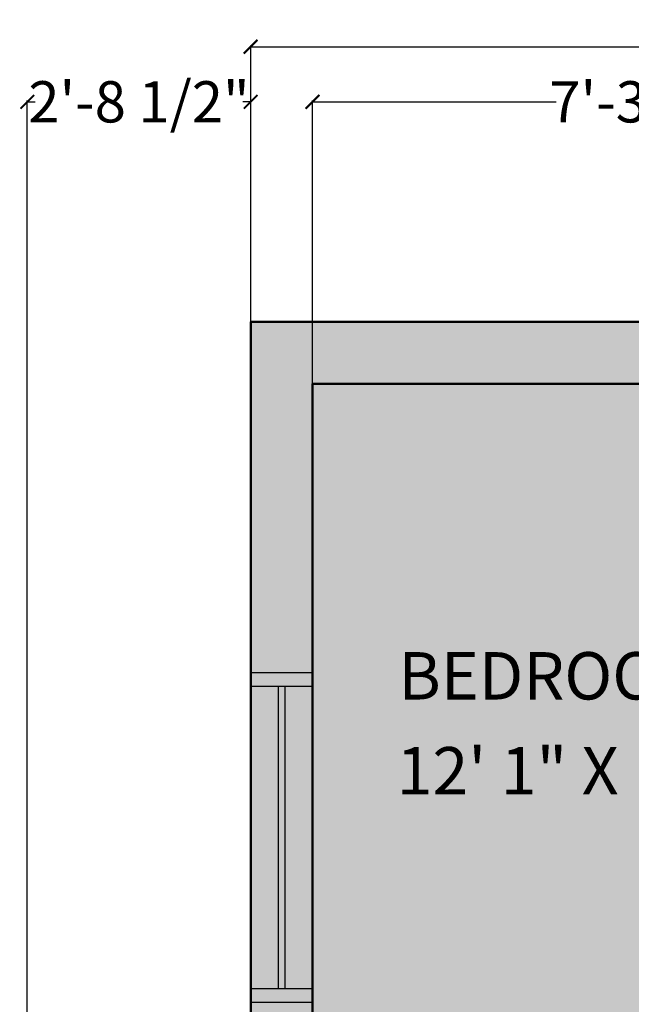
# Model space of a CAD drawing. Units: inches. Extents: x 528 to 2620, y -1066 to 798.
# Tile 26 of 41: x 1023 to 1112, y 620 to 763. Entities that reach past the tile are written whole.
import ezdxf

# ---------------------------------------------------------------- set-up
doc = ezdxf.new("R2010")
doc.units = ezdxf.units.IN
doc.header["$MEASUREMENT"] = 0
for name, color, linetype, lineweight in [('A-ANNO-DIMS', 2, 'Continuous', 18), ('A-AREA-IDEN', 7, 'Continuous', 18), ('A-GLAZ', 3, 'Continuous', 25), ('A-WALL', 7, 'Continuous', 50), ('A-WALL-PATT', 8, 'Continuous', 13)]:
    doc.layers.add(name, color=color, linetype=linetype, lineweight=lineweight)
doc.styles.get("Standard").update_dxf_attribs({"font": 'arial.ttf'})
doc.dimstyles.get("Standard").update_dxf_attribs({"dimtxt": 6, "dimasz": 2, "dimexe": 0.18, "dimexo": 0.0625, "dimgap": 0.09, "dimtad": 0, "dimtih": 1, "dimtoh": 1, "dimdec": 1, "dimzin": 0, "dimdsep": 46, "dimlunit": 3, "dimtxsty": 'Standard', "dimblk": 'ARCHTICK', "dimcen": 0.09, "dimadec": 0, "dimazin": 0, "dimtfac": 1, "dimtdec": 1, "dimtofl": 0, "dimtmove": 0, "dimatfit": 3, "dimfxl": 1, "dimtolj": 1, "dimtzin": 0, "dimarcsym": 0})

# ---------------------------------------------------------------- blocks, each defined once
blk = doc.blocks.new('_ArchTick')
at = {"color": 0, "linetype": 'ByBlock', "const_width": 0.15}
blk.add_lwpolyline([(-0.5, -0.5), (0.5, 0.5)], dxfattribs=at)
blk = doc.blocks.new('*D18')
at = {"layer": 'A-ANNO-DIMS', "color": 0, "lineweight": -2, "transparency": 16777216}
for p, q in [((1057, 718.98), (1057, 759.11)), ((1057, 758.93), (1195.76, 758.93)), ((1345, 758.93), (1206.23, 758.93)), ((1345, 718.98), (1345, 759.11))]:
    blk.add_line(p, q, dxfattribs=at)
at = {"layer": 'Defpoints', "color": 0, "transparency": 16777216}
for p in [(1345, 758.93), (1057, 718.92), (1345, 718.92)]:
    blk.add_point(p, dxfattribs=at)
at = {"layer": 'A-ANNO-DIMS', "color": 0, "lineweight": -2, "transparency": 16777216, "xscale": 2, "yscale": 2, "zscale": 2, "rotation": 180}
blk.add_blockref('_ArchTick', (1057, 758.93), dxfattribs=at)
at = {"layer": 'A-ANNO-DIMS', "color": 0, "lineweight": -2, "transparency": 16777216, "xscale": 2, "yscale": 2, "zscale": 2}
blk.add_blockref('_ArchTick', (1345, 758.93), dxfattribs=at)
at = {"layer": 'A-ANNO-DIMS', "color": 0, "transparency": 16777216, "insert": (1201, 758.93), "char_height": 6, "attachment_point": 5}
blk.add_mtext("\\A1;24'", dxfattribs=at)
blk = doc.blocks.new('WIN-1200')
for p, q in [((677.56, 718.92), (725.56, 718.92)), ((677.56, 709.92), (677.56, 718.92)), ((679.56, 709.92), (679.56, 718.92)), ((723.56, 718.92), (723.56, 709.92)), ((725.56, 718.92), (725.56, 709.92)), ((679.56, 714.92), (723.56, 714.92)), ((679.56, 713.92), (723.56, 713.92)), ((725.56, 709.92), (677.56, 709.92))]:
    blk.add_line(p, q)
blk = doc.blocks.new('*D63')
at = {"layer": 'A-ANNO-DIMS', "color": 0, "lineweight": -2, "transparency": 16777216}
for p, q in [((1024.5, 405.4), (1024.5, 751.1)), ((1024.5, 750.92), (1025.64, 750.92)), ((1057, 750.92), (1055.85, 750.92)), ((1057, 405.4), (1057, 751.1))]:
    blk.add_line(p, q, dxfattribs=at)
at = {"layer": 'Defpoints', "color": 0, "transparency": 16777216}
for p in [(1057, 750.92), (1024.5, 405.34), (1057, 405.34)]:
    blk.add_point(p, dxfattribs=at)
at = {"layer": 'A-ANNO-DIMS', "color": 0, "lineweight": -2, "transparency": 16777216, "xscale": 2, "yscale": 2, "zscale": 2, "rotation": 180}
blk.add_blockref('_ArchTick', (1024.5, 750.92), dxfattribs=at)
at = {"layer": 'A-ANNO-DIMS', "color": 0, "lineweight": -2, "transparency": 16777216, "xscale": 2, "yscale": 2, "zscale": 2}
blk.add_blockref('_ArchTick', (1057, 750.92), dxfattribs=at)
at = {"layer": 'A-ANNO-DIMS', "color": 0, "transparency": 16777216, "insert": (1040.75, 750.92), "char_height": 6, "attachment_point": 5}
blk.add_mtext('\\A1;2\'-8 1/2"', dxfattribs=at)
blk = doc.blocks.new('*D66')
at = {"layer": 'A-ANNO-DIMS', "color": 0, "lineweight": -2, "transparency": 16777216}
for p, q in [((1066, 400.48), (1066, 751.1)), ((1066, 750.92), (1101.46, 750.92)), ((1153, 750.92), (1117.54, 750.92)), ((1153, 400.48), (1153, 751.1))]:
    blk.add_line(p, q, dxfattribs=at)
at = {"layer": 'Defpoints', "color": 0, "transparency": 16777216}
for p in [(1153, 750.92), (1066, 400.42), (1153, 400.42)]:
    blk.add_point(p, dxfattribs=at)
at = {"layer": 'A-ANNO-DIMS', "color": 0, "lineweight": -2, "transparency": 16777216, "xscale": 2, "yscale": 2, "zscale": 2, "rotation": 180}
blk.add_blockref('_ArchTick', (1066, 750.92), dxfattribs=at)
at = {"layer": 'A-ANNO-DIMS', "color": 0, "lineweight": -2, "transparency": 16777216, "xscale": 2, "yscale": 2, "zscale": 2}
blk.add_blockref('_ArchTick', (1153, 750.92), dxfattribs=at)
at = {"layer": 'A-ANNO-DIMS', "color": 0, "transparency": 16777216, "insert": (1109.5, 750.92), "char_height": 6, "attachment_point": 5}
blk.add_mtext('\\A1;7\'-3"', dxfattribs=at)

msp = doc.modelspace()

# ---------------------------------------------------------------- hatches: boundary and pattern name
at = {"layer": 'A-WALL-PATT', "transparency": 33554521}
h = msp.add_hatch(color=256, dxfattribs=at)
h.dxf.hatch_style = 1
h.paths.add_polyline_path([(1066, 709.92), (1114.5, 709.92), (1114.5, 718.92), (1057, 718.92), (1057, 667.92), (1066, 667.92)])
h.paths.add_polyline_path([(1227.5, 718.92), (1162.5, 718.92), (1162.5, 709.92), (1211, 709.92), (1211, 577.92), (1205.42, 577.92), (1205.5, 573.42), (1211, 573.42), (1211, 567.42), (1215.5, 567.42), (1215.5, 669.42), (1268, 669.42), (1268, 675.92), (1263.5, 675.92), (1263.5, 673.92), (1215.5, 673.92), (1215.5, 709.92), (1227.5, 709.92)])
h.paths.add_polyline_path([(1345, 718.92), (1316, 718.92), (1316, 709.92), (1336, 709.92), (1336, 641.67), (1345, 641.67)])
h.paths.add_polyline_path([(1066, 619.92), (1057, 619.92), (1057, 561.42), (1066, 561.42), (1066, 573.42), (1161, 573.42), (1161, 569.42), (1165.5, 569.42), (1165.5, 577.92), (1066, 577.92)])
h.paths.add_polyline_path([(1216, 391.42), (1216, 400.42), (1207, 400.42), (1201, 400.42), (1201, 397.42), (1201, 391.42), (1207, 391.42), (1207, 268.92), (1252, 268.92), (1252, 277.92), (1216, 277.92), (1216, 359.77)])
h.paths.add_polyline_path([(1345, 395.92), (1336, 395.92), (1288, 395.92), (1288, 391.42), (1336, 391.42), (1336, 277.92), (1300, 277.92), (1300, 268.92), (1345, 268.92)])
h.paths.add_polyline_path([(1345, 593.67), (1336, 593.67), (1336, 525.42), (1215.5, 525.42), (1215.5, 527.17), (1211, 527.17), (1211, 520.92), (1336, 520.92), (1336, 443.92), (1345, 443.92)])
h.paths.add_polyline_path([(1066, 520.92), (1165.5, 520.92), (1165.5, 545.42), (1161, 545.42), (1161, 525.42), (1066, 525.42), (1066, 537.42), (1057, 537.42), (1057, 484.67), (1066, 484.67)])
h.paths.add_polyline_path([(1066, 436.67), (1057, 436.67), (1057, 391.42), (1085.5, 391.42), (1085.5, 400.42), (1066, 400.42)])
h.paths.add_polyline_path([(1153, 397.42), (1153, 400.42), (1133.5, 400.42), (1133.5, 391.42), (1153, 391.42)])
at = {"layer": 'A-WALL-PATT', "transparency": 33554681}
h = msp.add_hatch(color=256, dxfattribs=at)
h.dxf.hatch_style = 1
h.paths.add_polyline_path([(1062, 665.92), (1061, 665.92), (1061, 621.92), (1062, 621.92)])
h.paths.add_polyline_path([(1066, 667.92), (1057, 667.92), (1057, 665.92), (1066, 665.92)])
h.paths.add_polyline_path([(1066, 621.92), (1057, 621.92), (1057, 619.92), (1066, 619.92)])
h.paths.add_polyline_path([(1160.5, 714.92), (1116.5, 714.92), (1116.5, 713.92), (1160.5, 713.92)])
h.paths.add_polyline_path([(1162.5, 718.92), (1160.5, 718.92), (1160.5, 709.92), (1162.5, 709.92)])
h.paths.add_polyline_path([(1116.5, 718.92), (1114.5, 718.92), (1114.5, 709.92), (1116.5, 709.92)])
h.paths.add_polyline_path([(1251.5, 714.92), (1227.5, 714.92), (1227.5, 713.92), (1251.5, 713.92)])
h.paths.add_polyline_path([(1314, 714.92), (1270, 714.92), (1270, 713.92), (1314, 713.92)])
h.paths.add_polyline_path([(1316, 718.92), (1314, 718.92), (1314, 709.92), (1316, 709.92)])
h.paths.add_polyline_path([(1270, 718.92), (1268, 718.92), (1268, 709.92), (1270, 709.92)])
h.paths.add_polyline_path([(1087.5, 400.42), (1085.5, 400.42), (1085.5, 391.42), (1087.5, 391.42)])
h.paths.add_polyline_path([(1131.5, 396.42), (1087.5, 396.42), (1087.5, 395.42), (1131.5, 395.42)])
h.paths.add_polyline_path([(1133.5, 400.42), (1131.5, 400.42), (1131.5, 391.42), (1133.5, 391.42)])
h.paths.add_polyline_path([(1066, 438.67), (1057, 438.67), (1057, 436.67), (1066, 436.67)])
h.paths.add_polyline_path([(1066, 484.67), (1057, 484.67), (1057, 482.67), (1066, 482.67)])
h.paths.add_polyline_path([(1062, 482.67), (1061, 482.67), (1061, 438.67), (1062, 438.67)])
h = msp.add_hatch(color=256, dxfattribs=at)
h.dxf.hatch_style = 1
h.paths.add_polyline_path([(1066, 665.92), (1062, 665.92), (1062, 621.92), (1066, 621.92)])
h.paths.add_polyline_path([(1061, 665.92), (1057, 665.92), (1057, 621.92), (1061, 621.92)])
h.paths.add_polyline_path([(1160.5, 713.92), (1116.5, 713.92), (1116.5, 709.92), (1160.5, 709.92)])
h.paths.add_polyline_path([(1160.5, 718.92), (1116.5, 718.92), (1116.5, 714.92), (1160.5, 714.92)])
h.paths.add_polyline_path([(1251.5, 713.92), (1227.5, 713.92), (1227.5, 709.92), (1251.5, 709.92)])
h.paths.add_polyline_path([(1251.5, 718.92), (1227.5, 718.92), (1227.5, 714.92), (1251.5, 714.92)])
h.paths.add_polyline_path([(1314, 713.92), (1270, 713.92), (1270, 709.92), (1314, 709.92)])
h.paths.add_polyline_path([(1314, 718.92), (1270, 718.92), (1270, 714.92), (1314, 714.92)])
h.paths.add_polyline_path([(1345, 639.67), (1341, 639.67), (1341, 595.67), (1345, 595.67)])
h.paths.add_polyline_path([(1340, 639.67), (1336, 639.67), (1336, 595.67), (1340, 595.67)])
h.paths.add_polyline_path([(1345, 441.92), (1341, 441.92), (1341, 397.92), (1345, 397.92)])
h.paths.add_polyline_path([(1340, 441.92), (1336, 441.92), (1336, 397.92), (1340, 397.92)])
h.paths.add_polyline_path([(1298, 272.92), (1254, 272.92), (1254, 268.92), (1298, 268.92)])
h.paths.add_polyline_path([(1298, 277.92), (1254, 277.92), (1254, 273.92), (1298, 273.92)])
h.paths.add_polyline_path([(1131.5, 395.42), (1087.5, 395.42), (1087.5, 391.42), (1131.5, 391.42)])
h.paths.add_polyline_path([(1131.5, 400.42), (1087.5, 400.42), (1087.5, 396.42), (1131.5, 396.42)])
h.paths.add_polyline_path([(1066, 482.67), (1062, 482.67), (1062, 438.67), (1066, 438.67)])
h.paths.add_polyline_path([(1061, 482.67), (1057, 482.67), (1057, 438.67), (1061, 438.67)])
h.paths.add_polyline_path([(1066, 561.42), (1062, 561.42), (1062, 537.42), (1066, 537.42)])
h.paths.add_polyline_path([(1061, 561.42), (1057, 561.42), (1057, 537.42), (1061, 537.42)])
at = {"layer": 'A-WALL-PATT', "transparency": 33554536}
h = msp.add_hatch(color=256, dxfattribs=at)
h.dxf.hatch_style = 1
h.paths.add_polyline_path([(1336, 709.92), (1268, 709.92), (1268, 699.92), (1266.75, 699.92), (1266.75, 675.92), (1268, 675.92), (1268, 669.42), (1215.5, 669.42), (1215.5, 567.17), (1217, 567.17), (1257, 567.17), (1257, 565.42), (1256.96, 565.42, -0.401453), (1217, 527.17), (1215.5, 527.17), (1215.5, 525.42), (1336, 525.42)], flags=17)
h.paths.add_polyline_path([(1285.03, 635.93), (1285.23, 636.13), (1285.67, 636.26), (1286.21, 636.02), (1286.98, 636.08), (1332.98, 636.08), (1333.36, 636.22), (1333.82, 636.08), (1334.11, 635.71), (1334.11, 635.3), (1333.91, 634.86), (1333.82, 634.83), (1333.82, 592.74), (1333.97, 592.6), (1334.11, 592.29), (1334.11, 591.88), (1333.82, 591.51), (1333.36, 591.37), (1332.98, 591.51), (1332.64, 591.79), (1332.64, 591.51), (1286.98, 591.51), (1286.17, 591.67), (1286.07, 591.57), (1285.68, 591.37), (1285.23, 591.51), (1285.03, 591.71), (1284.83, 592.1), (1284.98, 592.54), (1285.13, 592.69), (1285.13, 634.95), (1284.98, 635.1), (1284.83, 635.54)], flags=16)
h.paths.add_polyline_path([(1285.03, 635.93), (1285.23, 636.13), (1285.67, 636.26), (1286.21, 636.02), (1286.98, 636.08), (1332.98, 636.08), (1333.36, 636.22), (1333.82, 636.08), (1334.11, 635.71), (1334.11, 635.3), (1333.97, 634.99), (1333.82, 634.85), (1333.82, 592.74), (1333.97, 592.6), (1334.11, 592.29), (1334.11, 591.88), (1333.82, 591.51), (1333.36, 591.37), (1332.98, 591.51), (1332.64, 591.79), (1332.64, 592.25), (1332.64, 635.35), (1332.64, 635.8), (1332.98, 636.08), (1312.23, 636.08), (1311.1, 635.48), (1310.63, 635.48), (1310.43, 635.23), (1309.94, 635.1), (1309.7, 634.99), (1309.06, 634.76), (1308.71, 634.61), (1308.32, 634.61), (1307.75, 634.36), (1307.11, 634.27), (1307.01, 634.11), (1306.77, 634.02), (1307.25, 633.28), (1306.87, 633.04), (1306.77, 632.88), (1306.37, 632.64), (1306.03, 632.55), (1305.54, 632.41), (1315.47, 618.49), (1316.32, 619.39), (1312.77, 622.86), (1319.62, 630.11), (1320.07, 629.68), (1320.11, 630), (1320.28, 630.6), (1320.53, 631.18), (1320.53, 632.01), (1320.26, 632.55), (1320.11, 633.13), (1320.06, 633.73), (1320.63, 634.02), (1321.22, 634.16), (1321.86, 634.11), (1322.45, 633.91), (1322.99, 633.62), (1324.1, 633.62), (1324.64, 633.91), (1325.23, 634.07), (1325.87, 634.07), (1326.43, 633.91), (1326.98, 633.62), (1328.35, 633.62), (1328.9, 633.91), (1329.49, 634.11), (1330.1, 634.16), (1330.69, 634.02), (1331.28, 633.73), (1331.23, 633.13), (1331.09, 632.55), (1330.79, 632.01), (1330.79, 631.18), (1331.04, 630.6), (1331.23, 630), (1331.28, 629.41), (1331.19, 628.79), (1331.04, 628.18), (1330.79, 627.6), (1330.79, 626.77), (1331.04, 626.19), (1331.23, 625.59), (1331.28, 625.01), (1331.19, 624.38), (1331.04, 623.78), (1330.79, 623.24), (1330.79, 622.37), (1331.04, 621.83), (1331.23, 621.25), (1331.28, 620.6), (1331.19, 619.97), (1331.04, 619.37), (1330.79, 618.83), (1330.79, 617.96), (1331.09, 617.42), (1331.23, 616.88), (1331.28, 616.23), (1331.28, 615.52), (1330.69, 615.27), (1330.1, 615.12), (1329.49, 615.12), (1328.9, 615.32), (1328.35, 615.65), (1326.98, 615.65), (1326.43, 615.32), (1325.87, 615.16), (1325.23, 615.16), (1324.64, 615.32), (1324.1, 615.65), (1323.24, 615.65), (1324.93, 614.04), (1322.98, 611.98), (1324.1, 611.98), (1324.64, 612.27), (1325.28, 612.43), (1325.87, 612.43), (1326.48, 612.27), (1327.03, 611.98), (1328.35, 611.98), (1328.9, 612.27), (1329.49, 612.48), (1330.1, 612.52), (1330.74, 612.39), (1331.28, 612.07), (1331.28, 611.36), (1331.28, 610.75), (1331.09, 610.17), (1330.79, 609.63), (1330.79, 608.81), (1331.09, 608.22), (1331.23, 607.62), (1331.28, 606.99), (1331.23, 606.41), (1331.09, 605.81), (1330.79, 605.22), (1330.79, 604.4), (1331.09, 603.81), (1331.23, 603.21), (1331.28, 602.63), (1331.23, 602), (1331.09, 601.4), (1330.79, 600.86), (1330.79, 599.99), (1331.09, 599.45), (1331.23, 598.87), (1331.28, 598.22), (1331.23, 597.59), (1331.09, 596.99), (1330.79, 596.45), (1330.79, 595.58), (1331.09, 595.04), (1331.28, 594.51), (1331.28, 593.86), (1330.74, 593.61), (1330.1, 593.48), (1329.49, 593.48), (1328.9, 593.68), (1328.35, 594.01), (1327.03, 594.01), (1326.48, 593.68), (1325.87, 593.52), (1325.28, 593.52), (1324.64, 593.68), (1324.1, 594.01), (1323.04, 594.01), (1322.5, 593.68), (1321.91, 593.48), (1321.27, 593.48), (1320.63, 593.61), (1320.11, 593.86), (1320.11, 594.51), (1320.28, 595.04), (1320.58, 595.58), (1320.58, 596.45), (1320.28, 596.99), (1320.16, 597.59), (1320.1, 598.01), (1319.62, 597.55), (1315.66, 601.73), (1312.23, 591.57), (1311.74, 591.66), (1311.59, 591.91), (1310.78, 592.4), (1309.55, 592.89), (1308.96, 592.89), (1308.71, 593.03), (1308.56, 593.14), (1307.75, 593.52), (1306.77, 593.61), (1307.25, 594.36), (1306.87, 594.6), (1306.37, 594.84), (1306.03, 595.09), (1305.54, 595.24), (1315.46, 609.35), (1310.93, 613.71), (1315.47, 618.49), (1305.54, 632.41), (1306.03, 632.55), (1306.37, 632.64), (1306.77, 632.88), (1306.87, 633.04), (1307.25, 633.28), (1306.77, 634.02), (1307.01, 634.11), (1307.11, 634.27), (1307.75, 634.36), (1308.32, 634.61), (1308.71, 634.61), (1309.06, 634.76), (1309.7, 634.99), (1309.94, 635.1), (1310.43, 635.23), (1310.63, 635.48), (1311.1, 635.48), (1312.23, 636.08), (1286.98, 636.08), (1286.22, 636.02), (1286.41, 635.44), (1286.21, 635.05), (1286.02, 634.85), (1285.87, 634.81), (1285.87, 592.84), (1286.15, 592.73), (1286.41, 592.19), (1286.23, 591.66), (1286.17, 591.67), (1286.07, 591.57), (1285.68, 591.37), (1285.23, 591.51), (1285.03, 591.71), (1284.83, 592.1), (1284.98, 592.54), (1285.13, 592.69), (1285.13, 634.95), (1284.98, 635.1), (1284.83, 635.54)], flags=0)
h.paths.add_polyline_path([(1322.5, 653.6), (1333.65, 653.6), (1333.65, 637.99), (1322.5, 637.99)], flags=16)
h.paths.add_polyline_path([(1323.62, 652.48), (1332.53, 652.48), (1332.53, 639.11), (1323.62, 639.11)], flags=0)
edge = h.paths.add_edge_path(flags=0)
edge.add_ellipse((1328.07, 645.79), major_axis=(2.24, 2.24), ratio=1, start_angle=405, end_angle=495, ccw=False)
edge.add_ellipse((1328.07, 645.79), major_axis=(2.24, 2.24), ratio=1, start_angle=675, end_angle=765, ccw=False)
edge.add_ellipse((1328.07, 645.79), major_axis=(2.24, 2.24), ratio=1, start_angle=585, end_angle=675, ccw=False)
edge.add_ellipse((1328.07, 645.79), major_axis=(2.24, 2.24), ratio=1, start_angle=495, end_angle=585, ccw=False)
h.paths.add_polyline_path([(1320.58, 628.39), (1320.33, 628.01), (1320.61, 628.55)], flags=0)
h.paths.add_polyline_path([(1317.89, 604.89), (1318.78, 604.64), (1319.76, 604.28), (1318.88, 604.53)], flags=0)
h.paths.add_polyline_path([(1320.33, 599.65), (1320.58, 599.25), (1320.58, 599.16)], flags=0)
h.paths.add_polyline_path([(1322.5, 589.6), (1333.65, 589.6), (1333.65, 573.99), (1322.5, 573.99)], flags=16)
h.paths.add_polyline_path([(1323.62, 588.48), (1332.53, 588.48), (1332.53, 575.11), (1323.62, 575.11)], flags=0)
edge = h.paths.add_edge_path(flags=0)
edge.add_ellipse((1328.07, 581.8), major_axis=(-2.24, 2.24), ratio=1, start_angle=-45, end_angle=45, ccw=False)
edge.add_ellipse((1328.07, 581.8), major_axis=(-2.24, 2.24), ratio=1, start_angle=-135, end_angle=-45, ccw=False)
edge.add_ellipse((1328.07, 581.8), major_axis=(-2.24, 2.24), ratio=1, start_angle=135, end_angle=-135, ccw=False)
edge.add_ellipse((1328.07, 581.8), major_axis=(-2.24, 2.24), ratio=1, start_angle=45, end_angle=135, ccw=False)
h.paths.add_polyline_path([(1264.75, 699.92), (1263.5, 699.92), (1263.5, 709.92), (1215.5, 709.92), (1215.5, 673.92), (1263.5, 673.92), (1263.5, 675.92), (1264.75, 675.92)], flags=16)
h.paths.add_polyline_path([(1162.19, 569.42), (1161, 569.42), (1161, 573.42), (1066, 573.42), (1066, 525.42), (1161, 525.42), (1161, 545.42), (1162.19, 545.42)])
h.paths.add_polyline_path([(1256.96, 565.42), (1257, 565.42), (1257, 567.17), (1217, 567.17), (1215.5, 567.17), (1215.5, 567.42), (1211, 567.42), (1211, 573.42), (1205.5, 573.42), (1205.42, 577.92), (1211, 577.92), (1211, 709.92), (1066, 709.92), (1066, 577.92), (1165.5, 577.92), (1165.5, 569.42), (1164.19, 569.42), (1164.19, 545.42), (1165.5, 545.42), (1165.5, 520.92), (1153, 520.92), (1153, 484.92), (1102, 484.92), (1102, 436.42), (1153, 436.42), (1153, 400.42), (1153, 391.42), (1201, 391.42), (1201, 400.42), (1207, 400.42), (1216, 400.42), (1216, 391.42), (1216, 277.92), (1336, 277.92), (1336, 391.42), (1288, 391.42), (1288, 395.92), (1336, 395.92), (1336, 443.92), (1336, 520.92), (1211, 520.92), (1211, 527.17), (1215.5, 527.17), (1217, 527.17, 0.401453)])
h.paths.add_polyline_path([(1167.25, 579.42), (1165.5, 579.42), (1165.5, 619.42), (1167.25, 619.42)], flags=16)
h.paths.add_polyline_path([(1227.97, 501.56), (1236.36, 502.03), (1236.36, 492.55), (1227.97, 493.02, -0.254069)], flags=16)
h.paths.add_polyline_path([(1243.34, 515.69, -0.254069), (1251.88, 515.69), (1252.35, 507.3), (1242.87, 507.3)], flags=16)
h.paths.add_polyline_path([(1239.18, 504.68), (1256.03, 504.68), (1256.03, 479.42), (1239.18, 479.42)], flags=16)
h.paths.add_polyline_path([(1227.97, 489.6), (1236.36, 490.07), (1236.36, 480.59), (1227.97, 481.06, -0.254069)], flags=16)
h.paths.add_polyline_path([(1197.2, 624.04), (1197.2, 639.64), (1208.35, 639.64), (1208.35, 624.04)], flags=16)
h.paths.add_polyline_path([(1198.32, 625.15), (1198.32, 638.53), (1207.23, 638.53), (1207.23, 625.15)], flags=0)
h.paths.add_polyline_path([(1258.85, 502.03), (1267.25, 501.56, -0.254069), (1267.25, 493.02), (1258.85, 492.55)], flags=16)
h.paths.add_polyline_path([(1271.59, 519.66), (1333.67, 519.66), (1333.67, 451.59), (1319.09, 451.59), (1319.09, 505.07), (1288.09, 505.07), (1284.45, 505.07, -0.883215), (1270.68, 514.19), (1270.68, 518.75, -0.414214)], flags=16)
h.paths.add_polyline_path([(1331.85, 517.83), (1331.85, 453.42), (1328.2, 453.42), (1328.2, 505.07), (1298.42, 505.07), (1298.42, 514.19), (1288.09, 514.19), (1288.09, 517.83)], flags=0)
h.paths.add_polyline_path([(1242.87, 476.8), (1252.35, 476.8), (1251.88, 468.41, -0.254069), (1243.34, 468.41)], flags=16)
h.paths.add_polyline_path([(1258.85, 490.07), (1267.25, 489.6, -0.254069), (1267.25, 481.06), (1258.85, 480.59)], flags=16)
h.paths.add_polyline_path([(1161.68, 641.55), (1160.87, 641.72), (1160.77, 641.62), (1160.38, 641.41), (1159.93, 641.55), (1159.73, 641.75), (1159.53, 642.14), (1159.68, 642.58), (1159.83, 642.73), (1159.83, 684.99), (1159.68, 685.14), (1159.53, 685.58), (1159.73, 685.97), (1159.93, 686.17), (1160.37, 686.31), (1160.91, 686.06), (1161.68, 686.13), (1207.68, 686.13), (1208.06, 686.27), (1208.52, 686.13), (1208.81, 685.76), (1208.81, 685.34), (1208.61, 684.9), (1208.52, 684.87), (1208.52, 642.78), (1208.67, 642.65), (1208.88, 642.2), (1208.72, 641.8), (1208.52, 641.55), (1208.06, 641.41), (1207.68, 641.55), (1207.34, 641.83), (1207.34, 641.55)], flags=16)
h.paths.add_polyline_path([(1186.93, 641.62), (1186.44, 641.71), (1186.29, 641.95), (1185.48, 642.45), (1184.25, 642.94), (1183.66, 642.94), (1183.41, 643.07), (1183.26, 643.18), (1182.45, 643.57), (1181.47, 643.65), (1181.95, 644.4), (1181.57, 644.64), (1181.07, 644.89), (1180.73, 645.13), (1180.24, 645.29), (1190.16, 659.4), (1185.63, 663.75), (1190.17, 668.54), (1180.24, 682.46), (1180.73, 682.59), (1181.07, 682.68), (1181.47, 682.93), (1181.57, 683.08), (1181.95, 683.33), (1181.47, 684.07), (1181.71, 684.16), (1181.81, 684.31), (1182.45, 684.4), (1183.02, 684.65), (1183.41, 684.65), (1183.76, 684.81), (1184.4, 685.03), (1184.64, 685.14), (1185.13, 685.28), (1185.33, 685.52), (1185.8, 685.52), (1186.93, 686.13), (1161.68, 686.13), (1160.92, 686.06), (1161.11, 685.49), (1160.91, 685.1), (1160.72, 684.9), (1160.57, 684.85), (1160.57, 642.88), (1160.85, 642.77), (1161.11, 642.23), (1160.93, 641.7), (1160.87, 641.72), (1160.77, 641.62), (1160.38, 641.41), (1159.93, 641.55), (1159.73, 641.75), (1159.53, 642.14), (1159.68, 642.58), (1159.83, 642.73), (1159.83, 684.99), (1159.68, 685.14), (1159.53, 685.58), (1159.73, 685.97), (1159.93, 686.17), (1160.37, 686.31), (1160.91, 686.06), (1161.68, 686.13), (1207.68, 686.13), (1208.06, 686.27), (1208.52, 686.13), (1208.81, 685.76), (1208.81, 685.34), (1208.67, 685.03), (1208.52, 684.9), (1208.52, 642.78), (1208.67, 642.65), (1208.88, 642.2), (1208.72, 641.8), (1208.52, 641.55), (1208.06, 641.41), (1207.68, 641.55), (1207.34, 641.83), (1207.34, 642.29), (1207.34, 685.39), (1207.34, 685.85), (1207.68, 686.13), (1186.93, 686.13), (1185.8, 685.52), (1185.33, 685.52), (1185.13, 685.28), (1184.64, 685.14), (1184.4, 685.03), (1183.76, 684.81), (1183.41, 684.65), (1183.02, 684.65), (1182.45, 684.4), (1181.81, 684.31), (1181.71, 684.16), (1181.47, 684.07), (1181.95, 683.33), (1181.57, 683.08), (1181.47, 682.93), (1181.07, 682.68), (1180.73, 682.59), (1180.24, 682.46), (1190.17, 668.54), (1191.02, 669.43), (1187.47, 672.9), (1194.32, 680.15), (1194.77, 679.72), (1194.81, 680.04), (1194.98, 680.65), (1195.23, 681.23), (1195.23, 682.05), (1194.96, 682.59), (1194.81, 683.17), (1194.76, 683.78), (1195.33, 684.07), (1195.92, 684.2), (1196.56, 684.16), (1197.15, 683.96), (1197.69, 683.67), (1198.8, 683.67), (1199.34, 683.96), (1199.93, 684.11), (1200.57, 684.11), (1201.13, 683.96), (1201.68, 683.67), (1203.05, 683.67), (1203.6, 683.96), (1204.19, 684.16), (1204.8, 684.2), (1205.39, 684.07), (1205.98, 683.78), (1205.93, 683.17), (1205.79, 682.59), (1205.49, 682.05), (1205.49, 681.23), (1205.74, 680.65), (1205.93, 680.04), (1205.98, 679.46), (1205.89, 678.83), (1205.74, 678.23), (1205.49, 677.65), (1205.49, 676.82), (1205.74, 676.24), (1205.93, 675.63), (1205.98, 675.05), (1205.89, 674.42), (1205.74, 673.82), (1205.49, 673.28), (1205.49, 672.41), (1205.74, 671.87), (1205.93, 671.29), (1205.98, 670.64), (1205.89, 670.02), (1205.74, 669.41), (1205.49, 668.87), (1205.49, 668), (1205.79, 667.46), (1205.93, 666.93), (1205.98, 666.28), (1205.98, 665.56), (1205.39, 665.32), (1204.8, 665.16), (1204.19, 665.16), (1203.6, 665.36), (1203.05, 665.7), (1201.68, 665.7), (1201.13, 665.36), (1200.57, 665.2), (1199.93, 665.2), (1199.34, 665.36), (1198.8, 665.7), (1197.94, 665.7), (1199.63, 664.09), (1197.68, 662.03), (1198.8, 662.03), (1199.34, 662.32), (1199.98, 662.47), (1200.57, 662.47), (1201.18, 662.32), (1201.73, 662.03), (1203.05, 662.03), (1203.6, 662.32), (1204.19, 662.52), (1204.8, 662.56), (1205.44, 662.43), (1205.98, 662.12), (1205.98, 661.4), (1205.98, 660.8), (1205.79, 660.21), (1205.49, 659.68), (1205.49, 658.85), (1205.79, 658.27), (1205.93, 657.66), (1205.98, 657.04), (1205.93, 656.45), (1205.79, 655.85), (1205.49, 655.27), (1205.49, 654.44), (1205.79, 653.86), (1205.93, 653.25), (1205.98, 652.67), (1205.93, 652.05), (1205.79, 651.44), (1205.49, 650.91), (1205.49, 650.03), (1205.79, 649.5), (1205.93, 648.91), (1205.98, 648.26), (1205.93, 647.64), (1205.79, 647.03), (1205.49, 646.5), (1205.49, 645.62), (1205.79, 645.09), (1205.98, 644.55), (1205.98, 643.9), (1205.44, 643.65), (1204.8, 643.52), (1204.19, 643.52), (1203.6, 643.72), (1203.05, 644.06), (1201.73, 644.06), (1201.18, 643.72), (1200.57, 643.57), (1199.98, 643.57), (1199.34, 643.72), (1198.8, 644.06), (1197.74, 644.06), (1197.2, 643.72), (1196.61, 643.52), (1195.97, 643.52), (1195.33, 643.65), (1194.81, 643.9), (1194.81, 644.55), (1194.98, 645.09), (1195.28, 645.62), (1195.28, 646.5), (1194.98, 647.03), (1194.86, 647.64), (1194.8, 648.06), (1194.32, 647.59), (1190.36, 651.77)], flags=16)
h.paths.add_polyline_path([(1195.28, 649.2), (1195.03, 649.7), (1195.28, 649.29)], flags=0)
h.paths.add_polyline_path([(1194.46, 654.33), (1193.58, 654.58), (1192.59, 654.93), (1193.48, 654.69)], flags=0)
h.paths.add_polyline_path([(1195.28, 678.43), (1195.03, 678.05), (1195.31, 678.59)], flags=0)
h.paths.add_polyline_path([(1197.2, 688.04), (1197.2, 703.64), (1208.35, 703.64), (1208.35, 688.04)], flags=16)
h.paths.add_polyline_path([(1198.32, 689.15), (1198.32, 702.53), (1207.23, 702.53), (1207.23, 689.15)], flags=0)
h.paths.add_polyline_path([(1217.1, 329.02), (1230.65, 329.02), (1230.65, 315.47), (1217.1, 315.47)], flags=16)
h.paths.add_polyline_path([(1223.87, 322.24), (1227.26, 322.24), (1227.26, 321.32, -0.414214), (1229.73, 318.86, -1), (1224.8, 318.86), (1223.87, 318.86)], flags=0)
h.paths.add_polyline_path([(1222.11, 325.63, -1), (1218.86, 325.63, -1)], flags=0)
h.paths.add_polyline_path([(1228.25, 325.63, -1), (1226.28, 325.63, -1)], flags=0)
h.paths.add_polyline_path([(1221.53, 318.86, -1), (1219.44, 318.86, -1)], flags=0)
h.paths.add_polyline_path([(1299.15, 293.73), (1299.15, 278.54), (1271.23, 278.54), (1271.23, 293.73)], flags=16)
h.paths.add_polyline_path([(1259.69, 292.21), (1270.62, 292.21, -1), (1270.62, 291.6), (1259.69, 291.6, -1)], flags=16)
h.paths.add_polyline_path([(1259.69, 291.3), (1270.62, 291.3, -1), (1270.62, 290.69), (1259.69, 290.69, -1)], flags=16)
h.paths.add_polyline_path([(1259.69, 290.39), (1270.62, 290.39, -1), (1270.62, 289.78), (1259.69, 289.78, -1)], flags=16)
h.paths.add_polyline_path([(1259.69, 289.48), (1270.62, 289.48, -1), (1270.62, 288.87), (1259.69, 288.87, -1)], flags=16)
h.paths.add_polyline_path([(1259.69, 288.57), (1270.62, 288.57, -1), (1270.62, 287.96), (1259.69, 287.96, -1)], flags=16)
h.paths.add_polyline_path([(1274.41, 292.38), (1283.25, 292.38, -0.414214), (1285.07, 290.56), (1285.07, 283.64, -0.414214), (1283.25, 281.82), (1277.72, 281.82), (1278.67, 280.87, -0.57735), (1279.38, 280.16), (1279.44, 280.11, -1), (1279.03, 279.7), (1278.97, 279.75, -0.57735), (1278.26, 280.46), (1276.9, 281.82), (1274.41, 281.82, -0.414214), (1272.58, 283.64), (1272.58, 290.56, -0.414214)], flags=0)
h.paths.add_polyline_path([(1259.69, 287.65), (1270.62, 287.65, -1), (1270.62, 287.05), (1259.69, 287.05, -1)], flags=16)
h.paths.add_polyline_path([(1259.69, 286.74), (1270.62, 286.74, -1), (1270.62, 286.14), (1259.69, 286.14, -1)], flags=16)
h.paths.add_polyline_path([(1259.69, 285.83), (1270.62, 285.83, -1), (1270.62, 285.22), (1259.69, 285.22, -1)], flags=16)
h.paths.add_polyline_path([(1259.69, 284.92), (1270.62, 284.92, -1), (1270.62, 284.31), (1259.69, 284.31, -1)], flags=16)
h.paths.add_polyline_path([(1259.69, 284.01), (1270.62, 284.01, -1), (1270.62, 283.4), (1259.69, 283.4, -1)], flags=16)
h.paths.add_polyline_path([(1287.82, 292.38), (1296.67, 292.38, -0.414214), (1298.49, 290.56), (1298.49, 283.64, -0.414214), (1296.67, 281.82), (1291.14, 281.82), (1292.09, 280.87, -0.57735), (1292.8, 280.16), (1292.85, 280.11, -1), (1292.44, 279.7), (1292.39, 279.75, -0.57735), (1291.68, 280.46), (1290.32, 281.82), (1287.82, 281.82, -0.414214), (1286, 283.64), (1286, 290.56, -0.414214)], flags=0)
h.paths.add_polyline_path([(1259.69, 283.1), (1270.62, 283.1, -1), (1270.62, 282.49), (1259.69, 282.49, -1)], flags=16)
h.paths.add_polyline_path([(1279.94, 287.61, -1), (1278.01, 287.61, -1)], flags=0)
h.paths.add_polyline_path([(1259.69, 282.19), (1270.62, 282.19, -1), (1270.62, 281.58), (1259.69, 281.58, -1)], flags=16)
h.paths.add_polyline_path([(1259.69, 281.27), (1270.62, 281.27, -1), (1270.62, 280.67), (1259.69, 280.67, -1)], flags=16)
h.paths.add_polyline_path([(1275.16, 284.17, -1), (1274.77, 284.17, -1)], flags=0)
h.paths.add_polyline_path([(1293.36, 287.61, -1), (1291.43, 287.61, -1)], flags=0)
h.paths.add_polyline_path([(1275.14, 280.5), (1276.33, 280.5, -5.828427), (1276.33, 280.12), (1275.14, 280.12, -1)], flags=0)
h.paths.add_polyline_path([(1288.57, 284.17, -1), (1288.19, 284.17, -1)], flags=0)
h.paths.add_polyline_path([(1281.31, 280.5), (1282.5, 280.5, -1), (1282.5, 280.12), (1281.31, 280.12, -5.828427)], flags=0)
h.paths.add_polyline_path([(1288.56, 280.5), (1289.75, 280.5, -5.828427), (1289.75, 280.12), (1288.56, 280.12, -1)], flags=0)
h.paths.add_polyline_path([(1294.73, 280.5), (1295.92, 280.5, -1), (1295.92, 280.12), (1294.73, 280.12, -5.828427)], flags=0)
h.paths.add_polyline_path([(1207, 391.42), (1201, 391.42), (1061.5, 391.42), (1061.5, 307.96), (1069, 307.96), (1069, 305.42), (1207, 305.42)])
at = {"layer": 'A-WALL-PATT', "transparency": 33554480}
h = msp.add_hatch(color=256, dxfattribs=at)
h.dxf.hatch_style = 1
h.paths.add_polyline_path([(1211, 709.92), (1066, 709.92), (1066, 577.92), (1165.5, 577.92), (1165.5, 579.42), (1165.5, 619.42), (1167.25, 619.42), (1167.25, 619.38, -0.401453), (1205.5, 579.42), (1205.5, 577.92), (1211, 577.92)])
h.paths.add_polyline_path([(1160.83, 686.06), (1160.91, 686.06), (1160.77, 686.13)], flags=16)
h.paths.add_polyline_path([(1160.93, 641.7), (1160.93, 641.71), (1160.93, 641.7)], flags=0)
h.paths.add_polyline_path([(1159.83, 684.99), (1159.58, 685.24), (1159.58, 685.82), (1160.02, 686.26), (1160.22, 686.26), (1159.93, 686.17), (1159.73, 685.97), (1159.58, 685.68), (1159.58, 685.43), (1159.68, 685.14), (1159.88, 684.94), (1160.17, 684.81), (1160.42, 684.81), (1160.72, 684.9), (1160.91, 685.1), (1161.11, 685.49), (1161.06, 685.64), (1161.06, 685.25), (1160.57, 684.75), (1160.57, 642.96), (1161.06, 642.51), (1161.06, 641.89), (1160.87, 641.72), (1161.68, 641.55), (1186.53, 641.55), (1186.29, 641.95), (1185.48, 642.45), (1184.25, 642.94), (1183.59, 642.94), (1183.26, 643.18), (1182.45, 643.57), (1181.47, 643.65), (1181.95, 644.4), (1181.57, 644.64), (1181.07, 644.89), (1180.73, 645.13), (1180.24, 645.29), (1190.16, 659.4), (1185.63, 663.75), (1190.17, 668.54), (1180.24, 682.46), (1180.73, 682.59), (1181.07, 682.68), (1181.47, 682.93), (1181.57, 683.08), (1181.95, 683.33), (1181.47, 684.07), (1181.71, 684.16), (1181.81, 684.31), (1182.45, 684.4), (1183.02, 684.65), (1183.41, 684.65), (1183.76, 684.81), (1184.4, 685.03), (1184.64, 685.14), (1185.13, 685.28), (1185.33, 685.52), (1185.8, 685.52), (1186.93, 686.13), (1207.68, 686.13), (1208.06, 686.27), (1208.63, 686.09), (1208.88, 685.48), (1208.61, 684.9), (1208.52, 684.87), (1208.52, 642.78), (1208.81, 642.51), (1208.81, 641.92), (1208.45, 641.46), (1207.79, 641.46), (1207.34, 641.83), (1207.34, 641.55), (1161.68, 641.55), (1160.93, 641.7), (1160.38, 641.41), (1159.82, 641.59), (1159.53, 642.14), (1159.72, 642.7), (1159.83, 642.76)], flags=16)
h.paths.add_polyline_path([(1159.83, 684.99), (1159.58, 685.24), (1159.58, 685.82), (1160.02, 686.26), (1160.22, 686.26), (1159.93, 686.17), (1159.73, 685.97), (1159.58, 685.68), (1159.58, 685.43), (1159.68, 685.14), (1159.83, 684.99), (1159.83, 642.73), (1159.68, 642.58), (1159.58, 642.29), (1159.58, 642.04), (1159.73, 641.75), (1160.02, 641.46), (1160.22, 641.46), (1159.82, 641.59), (1159.53, 642.14), (1159.68, 642.58), (1159.83, 642.73)], flags=0)
h.paths.add_polyline_path([(1207.68, 686.13), (1207.52, 686.13), (1207.49, 686.06)], flags=0)
h.paths.add_polyline_path([(1195.28, 648.71), (1195.29, 648.52), (1195.52, 648.75), (1195.52, 648.8), (1195.28, 649.2)], flags=0)
h.paths.add_polyline_path([(1194.77, 679.72), (1194.81, 680.04), (1194.98, 680.65), (1195.23, 681.23), (1195.23, 682.05), (1194.96, 682.59), (1194.81, 683.17), (1194.76, 683.78), (1195.33, 684.07), (1195.92, 684.2), (1196.56, 684.16), (1197.15, 683.96), (1197.69, 683.67), (1198.8, 683.67), (1199.34, 683.96), (1199.93, 684.11), (1200.57, 684.11), (1201.13, 683.96), (1201.68, 683.67), (1203.05, 683.67), (1203.6, 683.96), (1204.19, 684.16), (1204.8, 684.2), (1205.39, 684.07), (1205.98, 683.78), (1205.93, 683.17), (1205.79, 682.59), (1205.49, 682.05), (1205.49, 681.23), (1205.74, 680.65), (1205.93, 680.04), (1205.98, 679.46), (1205.89, 678.83), (1205.74, 678.23), (1205.49, 677.65), (1205.49, 676.82), (1205.74, 676.24), (1205.93, 675.63), (1205.98, 675.05), (1205.89, 674.42), (1205.74, 673.82), (1205.49, 673.28), (1205.49, 672.41), (1205.74, 671.87), (1205.93, 671.29), (1205.98, 670.64), (1205.89, 670.02), (1205.74, 669.41), (1205.49, 668.87), (1205.49, 668), (1205.79, 667.46), (1205.93, 666.93), (1205.98, 666.28), (1205.98, 665.56), (1205.39, 665.32), (1204.8, 665.16), (1204.19, 665.16), (1203.6, 665.36), (1203.05, 665.7), (1201.68, 665.7), (1201.13, 665.36), (1200.57, 665.2), (1199.93, 665.2), (1199.34, 665.36), (1198.8, 665.7), (1197.94, 665.7), (1199.63, 664.09), (1197.68, 662.03), (1198.8, 662.03), (1199.34, 662.32), (1199.98, 662.47), (1200.57, 662.47), (1201.18, 662.32), (1201.73, 662.03), (1203.05, 662.03), (1203.6, 662.32), (1204.19, 662.52), (1204.8, 662.56), (1205.44, 662.43), (1205.98, 662.12), (1205.98, 661.4), (1205.98, 660.8), (1205.79, 660.21), (1205.49, 659.68), (1205.49, 658.85), (1205.79, 658.27), (1205.93, 657.66), (1205.98, 657.04), (1205.93, 656.45), (1205.79, 655.85), (1205.49, 655.27), (1205.49, 654.44), (1205.79, 653.86), (1205.93, 653.25), (1205.98, 652.67), (1205.93, 652.05), (1205.79, 651.44), (1205.49, 650.91), (1205.49, 650.03), (1205.79, 649.5), (1205.93, 648.91), (1205.98, 648.26), (1205.93, 647.64), (1205.79, 647.03), (1205.49, 646.5), (1205.49, 645.62), (1205.79, 645.09), (1205.98, 644.55), (1205.98, 643.9), (1205.44, 643.65), (1204.8, 643.52), (1204.19, 643.52), (1203.6, 643.72), (1203.05, 644.06), (1201.73, 644.06), (1201.18, 643.72), (1200.57, 643.57), (1199.98, 643.57), (1199.34, 643.72), (1198.8, 644.06), (1197.74, 644.06), (1195.52, 644.3), (1205.29, 644.3), (1205.29, 661.45), (1197.13, 661.45), (1199.63, 664.09), (1196, 667.54), (1201.48, 673.28), (1195.52, 679), (1195.52, 678.92), (1195.31, 678.58), (1195.28, 678.43), (1195.03, 678.05), (1195.28, 678.52), (1195.28, 679.23)], flags=0)
h.paths.add_polyline_path([(1192.59, 654.93), (1193.48, 654.69), (1194.46, 654.33), (1193.58, 654.58)], flags=0)
h.paths.add_polyline_path([(1192.59, 672.79), (1193.43, 673.04), (1194.3, 673.35), (1194.29, 673.36), (1193.58, 673.15)], flags=0)
h.paths.add_polyline_path([(1195.28, 649.29), (1195.03, 649.7), (1195.3, 649.17)], flags=0)
h.paths.add_polyline_path([(1197.2, 639.64), (1208.35, 639.64), (1208.35, 624.04), (1197.2, 624.04)], flags=16)
h.paths.add_polyline_path([(1198.32, 638.53), (1207.23, 638.53), (1207.23, 625.15), (1198.32, 625.15)], flags=0)
edge = h.paths.add_edge_path(flags=0)
edge.add_ellipse((1202.77, 631.84), major_axis=(-2.24, 2.24), ratio=1, start_angle=-45, end_angle=45, ccw=False)
edge.add_ellipse((1202.77, 631.84), major_axis=(-2.24, 2.24), ratio=1, start_angle=-135, end_angle=-45, ccw=False)
edge.add_ellipse((1202.77, 631.84), major_axis=(-2.24, 2.24), ratio=1, start_angle=135, end_angle=-135, ccw=False)
edge.add_ellipse((1202.77, 631.84), major_axis=(-2.24, 2.24), ratio=1, start_angle=45, end_angle=135, ccw=False)
h.paths.add_polyline_path([(1197.2, 688.04), (1197.2, 703.64), (1208.35, 703.64), (1208.35, 688.04)], flags=16)
h.paths.add_polyline_path([(1198.32, 689.15), (1198.32, 702.53), (1207.23, 702.53), (1207.23, 689.15)], flags=0)
edge = h.paths.add_edge_path(flags=0)
edge.add_ellipse((1202.77, 695.84), major_axis=(2.24, 2.24), ratio=1, start_angle=405, end_angle=495, ccw=False)
edge.add_ellipse((1202.77, 695.84), major_axis=(2.24, 2.24), ratio=1, start_angle=675, end_angle=765, ccw=False)
edge.add_ellipse((1202.77, 695.84), major_axis=(2.24, 2.24), ratio=1, start_angle=585, end_angle=675, ccw=False)
edge.add_ellipse((1202.77, 695.84), major_axis=(2.24, 2.24), ratio=1, start_angle=495, end_angle=585, ccw=False)
h.paths.add_polyline_path([(1207.34, 685.39), (1207.34, 685.85), (1207.79, 686.22), (1208.45, 686.22), (1208.81, 685.76), (1208.81, 685.17), (1208.52, 684.9), (1208.52, 642.78), (1208.81, 642.51), (1208.81, 641.92), (1208.45, 641.46), (1207.79, 641.46), (1207.34, 641.83), (1207.34, 642.29)], flags=0)
h.paths.add_polyline_path([(1207.47, 642.68), (1207.99, 643.01), (1208.61, 642.77), (1208.88, 642.2), (1208.63, 641.59), (1208.06, 641.41), (1207.49, 641.62), (1207.28, 642.13)], flags=16)
h.paths.add_polyline_path([(1207.63, 684.9), (1207.88, 684.74), (1208.35, 684.74), (1208.67, 685.03), (1208.81, 685.34), (1208.81, 685.64), (1208.72, 685.88), (1208.45, 686.22), (1208.22, 686.22), (1208.63, 686.09), (1208.88, 685.48), (1208.67, 685.03), (1208.35, 684.74), (1207.79, 684.74)], flags=16)
h.paths.add_polyline_path([(1076.48, 648.31), (1137.07, 648.31), (1137.07, 658.87), (1076.48, 658.87)], flags=24)
h.paths.add_polyline_path([(1076.71, 662.1), (1130.01, 662.1), (1130.01, 672.8), (1076.71, 672.8)], flags=24)

# ---------------------------------------------------------------- linework, layer by layer
at = {"layer": 'A-WALL'}
for p, q in [((1345, 718.92), (1057, 718.92)), ((1057, 718.92), (1057, 391.42)), ((1211, 709.92), (1066, 709.92)), ((1066, 709.92), (1066, 577.92))]:
    msp.add_line(p, q, dxfattribs=at)

# ---------------------------------------------------------------- block references
at = {"layer": 'A-GLAZ', "rotation": 269.9999999999997}
msp.add_blockref('WIN-1200', (347.07, 1345.48), dxfattribs=at)

# ---------------------------------------------------------------- texts
at = {"layer": 'A-AREA-IDEN'}
for s, height, p in [('BEDROOM', 6.891, (1078.49, 664)), ('12\' 1" X 11\'0"', 6.8907, (1078.23, 650.19))]:
    msp.add_text(s, height=height, dxfattribs=at).set_placement(p)

# ---------------------------------------------------------------- dimensions: what is measured, and where the dimension line sits
at = {"layer": 'A-ANNO-DIMS'}
for base, p1, p2, override, picture, middle in [((1345, 758.93), (1057, 718.92), (1345, 718.92), {"dimclrd": 0, "dimclre": 0, "dimclrt": 0}, '*D18', (1201, 758.93)), ((1057, 750.92), (1024.5, 405.34), (1057, 405.34), {"dimdec": 1, "dimlfac": 1, "dimrnd": 0, "dimzin": 1, "dimdsep": 46, "dimlunit": 4, "dimfrac": 2}, '*D63', (1040.75, 750.92)), ((1153, 750.92), (1066, 400.42), (1153, 400.42), {"dimdec": 1, "dimlfac": 1, "dimrnd": 0, "dimzin": 1, "dimdsep": 46, "dimlunit": 4, "dimfrac": 2}, '*D66', (1109.5, 750.92))]:
    dim = msp.add_linear_dim(base=base, p1=p1, p2=p2, dimstyle='Standard', override=override, dxfattribs=at)
    dim.commit()
    dim.dimension.update_dxf_attribs({"geometry": picture, "text_midpoint": middle})

doc.saveas('drawing.dxf')
